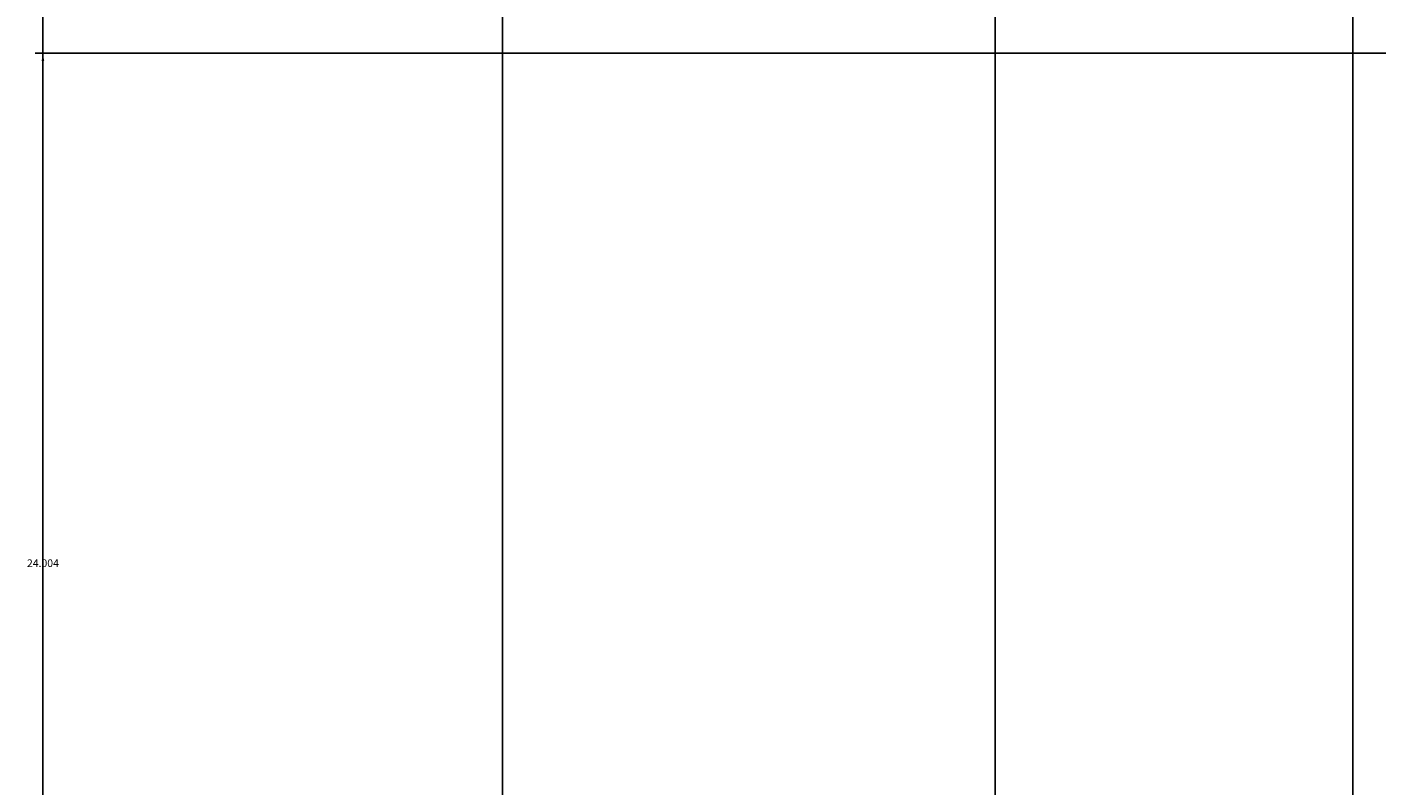
# Model space of a CAD drawing. Units: inches. Extents: x -117 to 121, y -77 to 40.
# Tile 10 of 45: x -117 to -85, y -5 to 12. Entities that reach past the tile are written whole.
import ezdxf

# ---------------------------------------------------------------- set-up
doc = ezdxf.new("R2010")
doc.units = ezdxf.units.IN
doc.header["$MEASUREMENT"] = 0
doc.layers.add('A-ANNO-DIMS', color=2, linetype='Continuous', lineweight=18)
doc.styles.get("Standard").update_dxf_attribs({"font": 'arial.ttf'})
doc.dimstyles.get("Standard").update_dxf_attribs({"dimtxt": 0.18, "dimasz": 0.18, "dimexe": 0.18, "dimexo": 0.0625, "dimgap": 0.09, "dimtad": 0, "dimtih": 1, "dimtoh": 1, "dimdec": 4, "dimzin": 0, "dimdsep": 46, "dimtxsty": 'Standard', "dimcen": 0.09, "dimadec": 0, "dimazin": 0, "dimtfac": 1, "dimtdec": 4, "dimtofl": 0, "dimtmove": 0, "dimatfit": 3, "dimfxl": 1, "dimtolj": 1, "dimtzin": 0, "dimarcsym": 0})

# ---------------------------------------------------------------- blocks, each defined once
blk = doc.blocks.new('*D13')
at = {"layer": 'A-ANNO-DIMS', "color": 0, "lineweight": -2, "transparency": 16777216}
for p, q in [((-2.663, 27.063), (-117.024, 27.063)), ((-116.844, 26.883), (-116.844, -16.974)), ((-116.844, -61.196), (-116.844, -17.338)), ((-106.096, -61.376), (-117.024, -61.376))]:
    blk.add_line(p, q, dxfattribs=at)
at = {"layer": 'A-ANNO-DIMS', "color": 0, "transparency": 16777216}
for points in [[(-116.874, 26.883), (-116.814, 26.883), (-116.844, 27.063)], [(-116.874, -61.196), (-116.814, -61.196), (-116.844, -61.376)]]:
    blk.add_solid(points, dxfattribs=at)
at = {"layer": 'Defpoints', "color": 0, "transparency": 16777216}
for p in [(-2.6, 27.063), (-116.844, -61.376), (-106.034, -61.376)]:
    blk.add_point(p, dxfattribs=at)
at = {"layer": 'A-ANNO-DIMS', "color": 0, "transparency": 16777216, "insert": (-116.844, -17.156), "char_height": 0.18, "attachment_point": 5}
blk.add_mtext('\\A1;88.44', dxfattribs=at)
blk = doc.blocks.new('*D20')
at = {"layer": 'A-ANNO-DIMS', "color": 0, "lineweight": -2, "transparency": 16777216}
for p, q in [((-75.866, 11.871), (-117.024, 11.871)), ((-116.844, 11.691), (-116.844, 0.051)), ((-116.844, -11.953), (-116.844, -0.313)), ((-94.498, -12.133), (-117.024, -12.133))]:
    blk.add_line(p, q, dxfattribs=at)
at = {"layer": 'A-ANNO-DIMS', "color": 0, "transparency": 16777216}
for points in [[(-116.874, 11.691), (-116.814, 11.691), (-116.844, 11.871)], [(-116.874, -11.953), (-116.814, -11.953), (-116.844, -12.133)]]:
    blk.add_solid(points, dxfattribs=at)
at = {"layer": 'Defpoints', "color": 0, "transparency": 16777216}
for p in [(-75.804, 11.871), (-116.844, -12.133), (-94.436, -12.133)]:
    blk.add_point(p, dxfattribs=at)
at = {"layer": 'A-ANNO-DIMS', "color": 0, "transparency": 16777216, "insert": (-116.844, -0.131), "char_height": 0.18, "attachment_point": 5}
blk.add_mtext('\\A1;24.004', dxfattribs=at)
blk = doc.blocks.new('*D21')
at = {"layer": 'A-ANNO-DIMS', "color": 0, "lineweight": -2, "transparency": 16777216}
for p, q in [((-106.034, -61.313), (-106.034, 38.61)), ((-75.804, 8.087), (-75.804, 38.61)), ((-105.854, 38.43), (-91.382, 38.43)), ((-75.984, 38.43), (-90.455, 38.43))]:
    blk.add_line(p, q, dxfattribs=at)
at = {"layer": 'A-ANNO-DIMS', "color": 0, "transparency": 16777216}
for points in [[(-105.854, 38.46), (-105.854, 38.4), (-106.034, 38.43)], [(-75.984, 38.46), (-75.984, 38.4), (-75.804, 38.43)]]:
    blk.add_solid(points, dxfattribs=at)
at = {"layer": 'Defpoints', "color": 0, "transparency": 16777216}
for p in [(-75.804, 38.43), (-75.804, 8.025), (-106.034, -61.376)]:
    blk.add_point(p, dxfattribs=at)
at = {"layer": 'A-ANNO-DIMS', "color": 0, "transparency": 16777216, "insert": (-90.919, 38.43), "char_height": 0.18, "attachment_point": 5}
blk.add_mtext('\\A1;30.230', dxfattribs=at)
blk = doc.blocks.new('*D39')
at = {"layer": 'A-ANNO-DIMS', "color": 0, "lineweight": -2, "transparency": 16777216}
for p, q in [((-94.436, -12.071), (-94.436, 38.61)), ((-86.023, -13.677), (-86.023, 38.61)), ((-94.256, 38.43), (-90.623, 38.43)), ((-86.203, 38.43), (-89.835, 38.43))]:
    blk.add_line(p, q, dxfattribs=at)
at = {"layer": 'A-ANNO-DIMS', "color": 0, "transparency": 16777216}
for points in [[(-94.256, 38.46), (-94.256, 38.4), (-94.436, 38.43)], [(-86.203, 38.46), (-86.203, 38.4), (-86.023, 38.43)]]:
    blk.add_solid(points, dxfattribs=at)
at = {"layer": 'Defpoints', "color": 0, "transparency": 16777216}
for p in [(-86.023, 38.43), (-94.436, -12.133), (-86.023, -13.74)]:
    blk.add_point(p, dxfattribs=at)
at = {"layer": 'A-ANNO-DIMS', "color": 0, "transparency": 16777216, "insert": (-90.229, 38.43), "char_height": 0.18, "attachment_point": 5}
blk.add_mtext('\\A1;8.413', dxfattribs=at)
blk = doc.blocks.new('*D40')
at = {"layer": 'A-ANNO-DIMS', "color": 0, "lineweight": -2, "transparency": 16777216}
for p, q in [((-86.023, -13.677), (-86.023, 38.61)), ((-63.159, -13.677), (-63.159, 38.61)), ((-85.843, 38.43), (-75.056, 38.43)), ((-63.339, 38.43), (-74.126, 38.43))]:
    blk.add_line(p, q, dxfattribs=at)
at = {"layer": 'A-ANNO-DIMS', "color": 0, "transparency": 16777216}
for points in [[(-85.843, 38.46), (-85.843, 38.4), (-86.023, 38.43)], [(-63.339, 38.46), (-63.339, 38.4), (-63.159, 38.43)]]:
    blk.add_solid(points, dxfattribs=at)
at = {"layer": 'Defpoints', "color": 0, "transparency": 16777216}
for p in [(-63.159, 38.43), (-86.023, -13.74), (-63.159, -13.74)]:
    blk.add_point(p, dxfattribs=at)
at = {"layer": 'A-ANNO-DIMS', "color": 0, "transparency": 16777216, "insert": (-74.591, 38.43), "char_height": 0.18, "attachment_point": 5}
blk.add_mtext('\\A1;22.864', dxfattribs=at)

msp = doc.modelspace()

# ---------------------------------------------------------------- dimensions: what is measured, and where the dimension line sits
at = {"layer": 'A-ANNO-DIMS'}
for base, p1, p2, picture, middle in [((-75.8037, 38.4297), (-106.0338, -61.3756), (-75.8037, 8.0246), '*D21', (-90.9187, 38.4297)), ((-86.0225, 38.4297), (-94.4355, -12.1334), (-86.0225, -13.74), '*D39', (-90.229, 38.4297)), ((-63.1589, 38.4297), (-86.0225, -13.74), (-63.1589, -13.74), '*D40', (-74.5907, 38.4297))]:
    dim = msp.add_linear_dim(base=base, p1=p1, p2=p2, dimstyle='Standard', override={"dimdec": 3, "dimlfac": 1, "dimrnd": 0, "dimzin": 0, "dimdsep": 46, "dimlunit": 2}, dxfattribs=at)
    dim.commit()
    dim.dimension.update_dxf_attribs({"geometry": picture, "text_midpoint": middle})
for base, p1, p2, override, picture, middle in [((-116.8438, -61.3756), (-2.6001, 27.0634), (-106.0338, -61.3756), {"dimdec": 2, "dimlfac": 1, "dimrnd": 0, "dimzin": 0, "dimdsep": 46, "dimlunit": 2}, '*D13', (-116.8438, -17.1561)), ((-116.84377, -12.13336), (-75.80372, 11.87111), (-94.43553, -12.13336), {"dimdec": 3, "dimlfac": 1, "dimrnd": 0, "dimzin": 0, "dimdsep": 46, "dimlunit": 2}, '*D20', (-116.84377, -0.13113))]:
    dim = msp.add_linear_dim(base=base, p1=p1, p2=p2, angle=90, dimstyle='Standard', override=override, dxfattribs=at)
    dim.commit()
    dim.dimension.update_dxf_attribs({"geometry": picture, "text_midpoint": middle})

doc.saveas('drawing.dxf')
